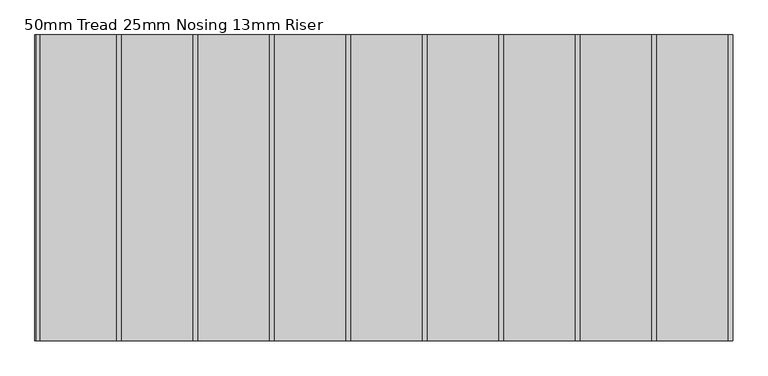
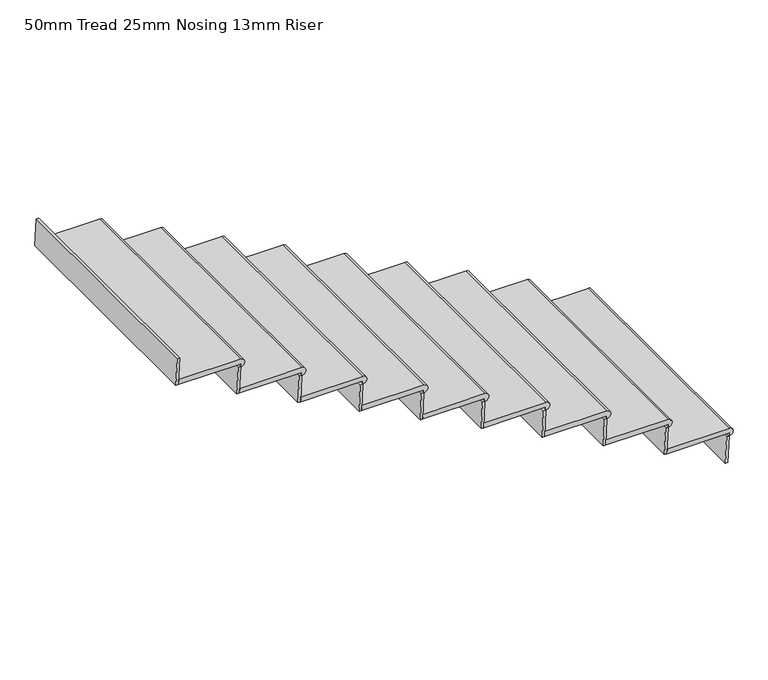
"""IFC4 building model written with IfcOpenShell, lengths in millimetres: stair flight geometry, 50mm Tread 25mm Nosing 13mm Riser."""

from ifc_helpers import new_model, si_unit, point, frame, frame_2d, origin, place, context, project, spatial, polyline, circle_curve, trimmed, segment, composite_curve, outline, extrude, source, transform, mapped, element, save


def stair_flight_50mm_tread_25mm_nosing_13mm_riser_e3034239(model_context):
    return source(origin(), model_context, "Body", "SweptSolid", [
        extrude(outline(composite_curve([segment(polyline([(1828.8, 9877.4583908), (1828.8, 9567.6583908), (1803.4, 9566.5284975), (1803.4, 9877.4583908), (1788.8, 9877.4583908)]), True, "CONTINUOUS"), segment(trimmed(circle_curve(frame_2d((1808.8, 9877.4583908)), 20.0), [point((1788.8, 9877.4583908))], [point((1828.8, 9877.4583908))], False, "CARTESIAN"), True, "CONTINUOUS")], self_intersect=False)), frame((0.0, 1038.0640673, 0.0), z_axis=(0.0, 1.0, 0.0), x_axis=(0.0, 0.0, 1.0)), (0.0, 0.0, 1.0), 1219.2),
        extrude(outline(polyline([(1788.8, 9877.4583908), (1788.8, 9864.9460292), (1651.0, 9858.816136), (1651.0, 9871.3284975), (1788.8, 9877.4583908)])), frame((0.0, 1038.0640673, 0.0), z_axis=(0.0, 1.0, 0.0), x_axis=(0.0, 0.0, 1.0)), (0.0, 0.0, 1.0), 1219.2),
        extrude(outline(polyline([(1941.2, 9572.6583908), (1941.2, 9560.1460292), (1803.4, 9554.016136), (1803.4, 9566.5284975), (1941.2, 9572.6583908)])), frame((0.0, 1038.0640673, 0.0), z_axis=(0.0, 1.0, 0.0), x_axis=(0.0, 0.0, 1.0)), (0.0, 0.0, 1.0), 1219.2),
        extrude(outline(composite_curve([segment(polyline([(1981.2, 9572.6583908), (1981.2, 9262.8583908), (1955.8, 9261.7284975), (1955.8, 9572.6583908), (1941.2, 9572.6583908)]), True, "CONTINUOUS"), segment(trimmed(circle_curve(frame_2d((1961.2, 9572.6583908)), 20.0), [point((1941.2, 9572.6583908))], [point((1981.2, 9572.6583908))], False, "CARTESIAN"), True, "CONTINUOUS")], self_intersect=False)), frame((0.0, 1038.0640673, 0.0), z_axis=(0.0, 1.0, 0.0), x_axis=(0.0, 0.0, 1.0)), (0.0, 0.0, 1.0), 1219.2),
        extrude(outline(polyline([(2093.6, 9267.8583908), (2093.6, 9255.3460292), (1955.8, 9249.216136), (1955.8, 9261.7284975), (2093.6, 9267.8583908)])), frame((0.0, 1038.0640673, 0.0), z_axis=(0.0, 1.0, 0.0), x_axis=(0.0, 0.0, 1.0)), (0.0, 0.0, 1.0), 1219.2),
        extrude(outline(composite_curve([segment(polyline([(2133.6, 9267.8583908), (2133.6, 8958.0583908), (2108.2, 8956.9284975), (2108.2, 9267.8583908), (2093.6, 9267.8583908)]), True, "CONTINUOUS"), segment(trimmed(circle_curve(frame_2d((2113.6, 9267.8583908)), 20.0), [point((2093.6, 9267.8583908))], [point((2133.6, 9267.8583908))], False, "CARTESIAN"), True, "CONTINUOUS")], self_intersect=False)), frame((0.0, 1038.0640673, 0.0), z_axis=(0.0, 1.0, 0.0), x_axis=(0.0, 0.0, 1.0)), (0.0, 0.0, 1.0), 1219.2),
        extrude(outline(polyline([(2246.0, 8963.0583908), (2246.0, 8950.5460292), (2108.2, 8944.416136), (2108.2, 8956.9284975), (2246.0, 8963.0583908)])), frame((0.0, 1038.0640673, 0.0), z_axis=(0.0, 1.0, 0.0), x_axis=(0.0, 0.0, 1.0)), (0.0, 0.0, 1.0), 1219.2),
        extrude(outline(composite_curve([segment(polyline([(2286.0, 8963.0583908), (2286.0, 8653.2583908), (2260.6, 8652.1284975), (2260.6, 8963.0583908), (2246.0, 8963.0583908)]), True, "CONTINUOUS"), segment(trimmed(circle_curve(frame_2d((2266.0, 8963.0583908)), 20.0), [point((2246.0, 8963.0583908))], [point((2286.0, 8963.0583908))], False, "CARTESIAN"), True, "CONTINUOUS")], self_intersect=False)), frame((0.0, 1038.0640673, 0.0), z_axis=(0.0, 1.0, 0.0), x_axis=(0.0, 0.0, 1.0)), (0.0, 0.0, 1.0), 1219.2),
        extrude(outline(polyline([(2398.4, 8658.2583908), (2398.4, 8645.7460292), (2260.6, 8639.616136), (2260.6, 8652.1284975), (2398.4, 8658.2583908)])), frame((0.0, 1038.0640673, 0.0), z_axis=(0.0, 1.0, 0.0), x_axis=(0.0, 0.0, 1.0)), (0.0, 0.0, 1.0), 1219.2),
        extrude(outline(composite_curve([segment(polyline([(2438.4, 8658.2583908), (2438.4, 8348.4583908), (2413.0, 8347.3284975), (2413.0, 8658.2583908), (2398.4, 8658.2583908)]), True, "CONTINUOUS"), segment(trimmed(circle_curve(frame_2d((2418.4, 8658.2583908)), 20.0), [point((2398.4, 8658.2583908))], [point((2438.4, 8658.2583908))], False, "CARTESIAN"), True, "CONTINUOUS")], self_intersect=False)), frame((0.0, 1038.0640673, 0.0), z_axis=(0.0, 1.0, 0.0), x_axis=(0.0, 0.0, 1.0)), (0.0, 0.0, 1.0), 1219.2),
        extrude(outline(polyline([(2550.8, 8353.4583908), (2550.8, 8340.9460292), (2413.0, 8334.816136), (2413.0, 8347.3284975), (2550.8, 8353.4583908)])), frame((0.0, 1038.0640673, 0.0), z_axis=(0.0, 1.0, 0.0), x_axis=(0.0, 0.0, 1.0)), (0.0, 0.0, 1.0), 1219.2),
        extrude(outline(composite_curve([segment(polyline([(2590.8, 8353.4583908), (2590.8, 8043.6583908), (2565.4, 8042.5284975), (2565.4, 8353.4583908), (2550.8, 8353.4583908)]), True, "CONTINUOUS"), segment(trimmed(circle_curve(frame_2d((2570.8, 8353.4583908)), 20.0), [point((2550.8, 8353.4583908))], [point((2590.8, 8353.4583908))], False, "CARTESIAN"), True, "CONTINUOUS")], self_intersect=False)), frame((0.0, 1038.0640673, 0.0), z_axis=(0.0, 1.0, 0.0), x_axis=(0.0, 0.0, 1.0)), (0.0, 0.0, 1.0), 1219.2),
        extrude(outline(polyline([(2703.2, 8048.6583908), (2703.2, 8036.1460292), (2565.4, 8030.016136), (2565.4, 8042.5284975), (2703.2, 8048.6583908)])), frame((0.0, 1038.0640673, 0.0), z_axis=(0.0, 1.0, 0.0), x_axis=(0.0, 0.0, 1.0)), (0.0, 0.0, 1.0), 1219.2),
        extrude(outline(composite_curve([segment(polyline([(2743.2, 8048.6583908), (2743.2, 7738.8583908), (2717.8, 7737.7284975), (2717.8, 8048.6583908), (2703.2, 8048.6583908)]), True, "CONTINUOUS"), segment(trimmed(circle_curve(frame_2d((2723.2, 8048.6583908)), 20.0), [point((2703.2, 8048.6583908))], [point((2743.2, 8048.6583908))], False, "CARTESIAN"), True, "CONTINUOUS")], self_intersect=False)), frame((0.0, 1038.0640673, 0.0), z_axis=(0.0, 1.0, 0.0), x_axis=(0.0, 0.0, 1.0)), (0.0, 0.0, 1.0), 1219.2),
        extrude(outline(polyline([(2855.6, 7743.8583908), (2855.6, 7731.3460292), (2717.8, 7725.216136), (2717.8, 7737.7284975), (2855.6, 7743.8583908)])), frame((0.0, 1038.0640673, 0.0), z_axis=(0.0, 1.0, 0.0), x_axis=(0.0, 0.0, 1.0)), (0.0, 0.0, 1.0), 1219.2),
        extrude(outline(composite_curve([segment(polyline([(2895.6, 7743.8583908), (2895.6, 7434.0583908), (2870.2, 7432.9284975), (2870.2, 7743.8583908), (2855.6, 7743.8583908)]), True, "CONTINUOUS"), segment(trimmed(circle_curve(frame_2d((2875.6, 7743.8583908)), 20.0), [point((2855.6, 7743.8583908))], [point((2895.6, 7743.8583908))], False, "CARTESIAN"), True, "CONTINUOUS")], self_intersect=False)), frame((0.0, 1038.0640673, 0.0), z_axis=(0.0, 1.0, 0.0), x_axis=(0.0, 0.0, 1.0)), (0.0, 0.0, 1.0), 1219.2),
        extrude(outline(polyline([(3008.0, 7439.0583908), (3008.0, 7426.5460292), (2870.2, 7420.416136), (2870.2, 7432.9284975), (3008.0, 7439.0583908)])), frame((0.0, 1038.0640673, 0.0), z_axis=(0.0, 1.0, 0.0), x_axis=(0.0, 0.0, 1.0)), (0.0, 0.0, 1.0), 1219.2),
        extrude(outline(polyline([(3160.4, 7134.2583908), (3160.4, 7121.7460292), (3022.6, 7115.616136), (3022.6, 7128.1284975), (3160.4, 7134.2583908)])), frame((0.0, 1038.0640673, 0.0), z_axis=(0.0, 1.0, 0.0), x_axis=(0.0, 0.0, 1.0)), (0.0, 0.0, 1.0), 1219.2),
        extrude(outline(composite_curve([segment(polyline([(3048.0, 7439.0583908), (3048.0, 7129.2583908), (3022.6, 7128.1284975), (3022.6, 7439.0583908), (3008.0, 7439.0583908)]), True, "CONTINUOUS"), segment(trimmed(circle_curve(frame_2d((3028.0, 7439.0583908)), 20.0), [point((3008.0, 7439.0583908))], [point((3048.0, 7439.0583908))], False, "CARTESIAN"), True, "CONTINUOUS")], self_intersect=False)), frame((0.0, 1038.0640673, 0.0), z_axis=(0.0, 1.0, 0.0), x_axis=(0.0, 0.0, 1.0)), (0.0, 0.0, 1.0), 1219.2),
    ])


if __name__ == "__main__":
    model = new_model("IFC4")
    model_context = context("Model", 3, world=origin())
    ifc_project = project(units=[si_unit("LENGTHUNIT", "METRE", prefix="MILLI")], contexts=[model_context])
    site = spatial("IfcSite", under=ifc_project)
    building = spatial("IfcBuilding", under=site)
    placement = place(None, origin())
    stair_flight_50mm_tread_25mm_nosing_13mm_riser_shape = stair_flight_50mm_tread_25mm_nosing_13mm_riser_e3034239(model_context)
    element("IfcStairFlight", 1, ObjectType="50mm Tread 25mm Nosing 13mm Riser", at=placement, inside=building, context=model_context, shape_type="MappedRepresentation", body=[
        mapped(stair_flight_50mm_tread_25mm_nosing_13mm_riser_shape, transform((0.0, 0.0, 0.0), x_axis=(1.0, 0.0, 0.0), y_axis=(0.0, 1.0, 0.0), z_axis=(0.0, 0.0, 1.0))),
    ])
    save(model, "model.ifc")
